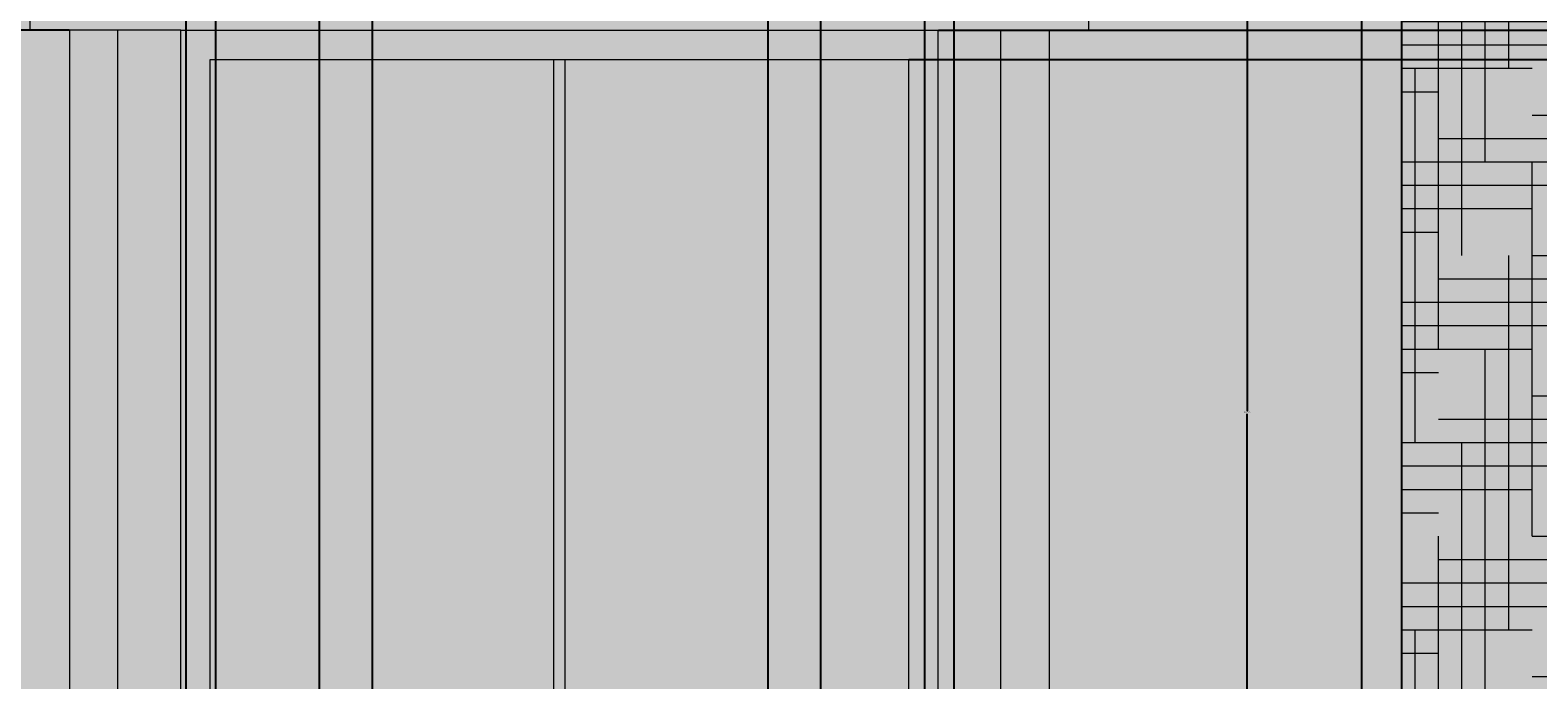
# Model space of a CAD drawing. Units: inches. Extents: x 3024 to 4744, y 1110 to 2100.
# Tile 23 of 29: x 3149 to 3354, y 1809 to 1897. Entities that reach past the tile are written whole.
import ezdxf

# ---------------------------------------------------------------- set-up
doc = ezdxf.new("R2010")
doc.units = ezdxf.units.IN
for name, color, linetype, lineweight in [('A-ANNO-DIMS', 2, 'Continuous', 18), ('A-ELEV', 7, 'Continuous', 25), ('A-ELEV-PATT', 252, 'Continuous', 13), ('A-GLAZ', 4, 'Continuous', 18)]:
    doc.layers.add(name, color=color, linetype=linetype, lineweight=lineweight)
doc.styles.get("Standard").update_dxf_attribs({"font": 'arial.ttf'})
doc.dimstyles.get("Standard").update_dxf_attribs({"dimtxt": 0.18, "dimasz": 0.18, "dimexe": 0.18, "dimexo": 0.0625, "dimgap": 0.09, "dimtad": 0, "dimtih": 1, "dimtoh": 1, "dimdec": 1, "dimzin": 0, "dimdsep": 46, "dimlunit": 3, "dimtxsty": 'Standard', "dimcen": 0.09, "dimadec": 0, "dimazin": 0, "dimtfac": 1, "dimtdec": 1, "dimtofl": 0, "dimtmove": 0, "dimatfit": 3, "dimfxl": 1, "dimtolj": 1, "dimtzin": 0, "dimarcsym": 0})

# ---------------------------------------------------------------- blocks, each defined once
blk = doc.blocks.new('WIN-BALCONY-A')
for p, q in [((3169.4, 1897.49), (3148.97, 1897.49)), ((3169.4, 1897.49), (3148.97, 1897.49)), ((3169.4, 1897.49), (3292.61, 1897.49)), ((3169.4, 1897.49), (3292.61, 1897.49)), ((3169.4, 1795.04), (3148.97, 1795.04)), ((3169.4, 1795.04), (3148.97, 1795.04)), ((3169.4, 1795.04), (3292.61, 1795.04)), ((3169.4, 1795.04), (3292.61, 1795.04))]:
    blk.add_line(p, q)
for points in [[(3148.97, 1897.49), (3148.97, 1905.61), (3292.61, 1905.61), (3292.61, 1897.49)], [(3148.97, 1897.49), (3148.97, 1905.61), (3292.61, 1905.61), (3292.61, 1897.49)], [(3292.61, 1795.04), (3292.61, 1785.61), (3148.97, 1785.61), (3148.97, 1795.04)], [(3292.61, 1795.04), (3292.61, 1785.61), (3148.97, 1785.61), (3148.97, 1795.04)]]:
    blk.add_lwpolyline(points)
for points in [[(3154.33, 1806.87), (3160.86, 1806.87), (3160.86, 1897.49), (3154.33, 1897.49)], [(3154.33, 1806.87), (3160.86, 1806.87), (3160.86, 1897.49), (3154.33, 1897.49)], [(3272.18, 1795.04), (3169.4, 1795.04), (3169.4, 1897.49), (3272.18, 1897.49)], [(3272.18, 1795.04), (3169.4, 1795.04), (3169.4, 1897.49), (3272.18, 1897.49)], [(3287.25, 1806.87), (3280.72, 1806.87), (3280.72, 1897.49), (3287.25, 1897.49)], [(3287.25, 1806.87), (3280.72, 1806.87), (3280.72, 1897.49), (3287.25, 1897.49)], [(3268.18, 1799.04), (3173.4, 1799.04), (3173.4, 1893.49), (3268.18, 1893.49)], [(3268.18, 1799.04), (3173.4, 1799.04), (3173.4, 1893.49), (3268.18, 1893.49)], [(3220.05, 1893.49), (3221.52, 1893.49), (3221.52, 1799.04), (3220.05, 1799.04)], [(3220.05, 1893.49), (3221.52, 1893.49), (3221.52, 1799.04), (3220.05, 1799.04)], [(3163.53, 1795.04), (3151.66, 1795.04), (3151.66, 1806.87), (3163.53, 1806.87)], [(3163.53, 1795.04), (3151.66, 1795.04), (3151.66, 1806.87), (3163.53, 1806.87)], [(3276.51, 1795.04), (3288.38, 1795.04), (3288.38, 1806.87), (3276.51, 1806.87)], [(3276.51, 1795.04), (3288.38, 1795.04), (3288.38, 1806.87), (3276.51, 1806.87)]]:
    blk.add_lwpolyline(points, close=True)
blk = doc.blocks.new('*D7')
at = {"layer": 'A-ANNO-DIMS', "color": 0, "lineweight": -2, "transparency": 16777216}
for p, q in [((3292.67, 1905.61), (3314.33, 1905.61)), ((3314.15, 1905.43), (3314.15, 1845.79)), ((3314.15, 1785.79), (3314.15, 1845.43)), ((3292.67, 1785.61), (3314.33, 1785.61))]:
    blk.add_line(p, q, dxfattribs=at)
at = {"layer": 'A-ANNO-DIMS', "color": 0, "transparency": 16777216}
for points in [[(3314.12, 1905.43), (3314.18, 1905.43), (3314.15, 1905.61)], [(3314.12, 1785.79), (3314.18, 1785.79), (3314.15, 1785.61)]]:
    blk.add_solid(points, dxfattribs=at)
at = {"layer": 'Defpoints', "color": 0, "transparency": 16777216}
for p in [(3292.61, 1905.61), (3314.15, 1905.61), (3292.61, 1785.61)]:
    blk.add_point(p, dxfattribs=at)
at = {"layer": 'A-ANNO-DIMS', "color": 0, "transparency": 16777216, "insert": (3314.15, 1845.61), "char_height": 0.18, "attachment_point": 5}
blk.add_mtext('\\A1;120 TYP.', dxfattribs=at)
blk = doc.blocks.new('*D64')
at = {"layer": 'A-ANNO-DIMS', "color": 0, "lineweight": -2, "transparency": 16777216}
for p, q in [((3069.79, 1241.5), (3069.79, 2100.44)), ((3069.97, 2100.26), (3405.08, 2100.26)), ((3740.97, 2100.26), (3405.87, 2100.26)), ((3741.15, 1241.5), (3741.15, 2100.44))]:
    blk.add_line(p, q, dxfattribs=at)
at = {"layer": 'A-ANNO-DIMS', "color": 0, "transparency": 16777216}
for points in [[(3069.97, 2100.29), (3069.97, 2100.23), (3069.79, 2100.26)], [(3740.97, 2100.29), (3740.97, 2100.23), (3741.15, 2100.26)]]:
    blk.add_solid(points, dxfattribs=at)
at = {"layer": 'Defpoints', "color": 0, "transparency": 16777216}
for p in [(3741.15, 2100.26), (3069.79, 1241.43), (3741.15, 1241.43)]:
    blk.add_point(p, dxfattribs=at)
at = {"layer": 'A-ANNO-DIMS', "color": 0, "transparency": 16777216, "insert": (3405.47, 2100.26), "char_height": 0.18, "attachment_point": 5}
blk.add_mtext('\\A1;671.4', dxfattribs=at)
blk = doc.blocks.new('*D98')
at = {"layer": 'A-ANNO-DIMS', "color": 0, "lineweight": -2, "transparency": 16777216}
for p, q in [((3154.27, 1897.49), (3024.11, 1897.49)), ((3024.29, 1897.31), (3024.29, 1852.36)), ((3024.29, 1807.05), (3024.29, 1852)), ((3154.27, 1806.87), (3024.11, 1806.87))]:
    blk.add_line(p, q, dxfattribs=at)
at = {"layer": 'A-ANNO-DIMS', "color": 0, "transparency": 16777216}
for points in [[(3024.26, 1897.31), (3024.32, 1897.31), (3024.29, 1897.49)], [(3024.26, 1807.05), (3024.32, 1807.05), (3024.29, 1806.87)]]:
    blk.add_solid(points, dxfattribs=at)
at = {"layer": 'Defpoints', "color": 0, "transparency": 16777216}
for p in [(3024.29, 1897.49), (3154.33, 1897.49), (3154.33, 1806.87)]:
    blk.add_point(p, dxfattribs=at)
at = {"layer": 'A-ANNO-DIMS', "color": 0, "transparency": 16777216, "insert": (3024.29, 1852.18), "char_height": 0.18, "attachment_point": 5}
blk.add_mtext('\\A1;90.62', dxfattribs=at)
blk = doc.blocks.new('*D101')
at = {"layer": 'A-ANNO-DIMS', "color": 0, "lineweight": -2, "transparency": 16777216}
for p, q in [((3268.24, 1893.49), (3786.83, 1893.49)), ((3786.65, 1893.31), (3786.65, 1846.45)), ((3786.65, 1799.22), (3786.65, 1846.08)), ((3268.24, 1799.04), (3786.83, 1799.04))]:
    blk.add_line(p, q, dxfattribs=at)
at = {"layer": 'A-ANNO-DIMS', "color": 0, "transparency": 16777216}
for points in [[(3786.62, 1893.31), (3786.68, 1893.31), (3786.65, 1893.49)], [(3786.62, 1799.22), (3786.68, 1799.22), (3786.65, 1799.04)]]:
    blk.add_solid(points, dxfattribs=at)
at = {"layer": 'Defpoints', "color": 0, "transparency": 16777216}
for p in [(3268.18, 1893.49), (3786.65, 1893.49), (3268.18, 1799.04)]:
    blk.add_point(p, dxfattribs=at)
at = {"layer": 'A-ANNO-DIMS', "color": 0, "transparency": 16777216, "insert": (3786.65, 1846.27), "char_height": 0.18, "attachment_point": 5}
blk.add_mtext('\\A1;94.44', dxfattribs=at)
blk = doc.blocks.new('*D102')
at = {"layer": 'A-ANNO-DIMS', "color": 0, "lineweight": -2, "transparency": 16777216}
for p, q in [((3272.24, 1897.49), (3786.83, 1897.49)), ((3786.65, 1897.31), (3786.65, 1895.67)), ((3786.65, 1893.67), (3786.65, 1895.31)), ((3268.24, 1893.49), (3786.83, 1893.49))]:
    blk.add_line(p, q, dxfattribs=at)
at = {"layer": 'A-ANNO-DIMS', "color": 0, "transparency": 16777216}
for points in [[(3786.62, 1897.31), (3786.68, 1897.31), (3786.65, 1897.49)], [(3786.62, 1893.67), (3786.68, 1893.67), (3786.65, 1893.49)]]:
    blk.add_solid(points, dxfattribs=at)
at = {"layer": 'Defpoints', "color": 0, "transparency": 16777216}
for p in [(3272.18, 1897.49), (3786.65, 1897.49), (3268.18, 1893.49)]:
    blk.add_point(p, dxfattribs=at)
at = {"layer": 'A-ANNO-DIMS', "color": 0, "transparency": 16777216, "insert": (3786.65, 1895.49), "char_height": 0.18, "attachment_point": 5}
blk.add_mtext('\\A1;4.00', dxfattribs=at)
blk = doc.blocks.new('*D106')
at = {"layer": 'A-ANNO-DIMS', "color": 0, "lineweight": -2, "transparency": 16777216}
for p, q in [((3170.16, 1275.67), (3170.16, 2100.44)), ((3170.34, 2100.26), (3171.83, 2100.26)), ((3173.98, 2100.26), (3172.49, 2100.26)), ((3174.16, 1271.67), (3174.16, 2100.44))]:
    blk.add_line(p, q, dxfattribs=at)
at = {"layer": 'A-ANNO-DIMS', "color": 0, "transparency": 16777216}
for points in [[(3170.34, 2100.29), (3170.34, 2100.23), (3170.16, 2100.26)], [(3173.98, 2100.29), (3173.98, 2100.23), (3174.16, 2100.26)]]:
    blk.add_solid(points, dxfattribs=at)
at = {"layer": 'Defpoints', "color": 0, "transparency": 16777216}
for p in [(3174.16, 2100.26), (3170.16, 1275.61), (3174.16, 1271.61)]:
    blk.add_point(p, dxfattribs=at)
at = {"layer": 'A-ANNO-DIMS', "color": 0, "transparency": 16777216, "insert": (3172.16, 2100.26), "char_height": 0.18, "attachment_point": 5}
blk.add_mtext('\\A1;4.00', dxfattribs=at)
blk = doc.blocks.new('*D107')
at = {"layer": 'A-ANNO-DIMS', "color": 0, "lineweight": -2, "transparency": 16777216}
for p, q in [((3174.16, 1271.67), (3174.16, 2100.44)), ((3174.34, 2100.26), (3221.88, 2100.26)), ((3270.21, 2100.26), (3222.67, 2100.26)), ((3270.39, 1271.67), (3270.39, 2100.44))]:
    blk.add_line(p, q, dxfattribs=at)
at = {"layer": 'A-ANNO-DIMS', "color": 0, "transparency": 16777216}
for points in [[(3174.34, 2100.29), (3174.34, 2100.23), (3174.16, 2100.26)], [(3270.21, 2100.29), (3270.21, 2100.23), (3270.39, 2100.26)]]:
    blk.add_solid(points, dxfattribs=at)
at = {"layer": 'Defpoints', "color": 0, "transparency": 16777216}
for p in [(3270.39, 2100.26), (3174.16, 1271.61), (3270.39, 1271.61)]:
    blk.add_point(p, dxfattribs=at)
at = {"layer": 'A-ANNO-DIMS', "color": 0, "transparency": 16777216, "insert": (3222.27, 2100.26), "char_height": 0.18, "attachment_point": 5}
blk.add_mtext('\\A1;96.23', dxfattribs=at)
blk = doc.blocks.new('*D108')
at = {"layer": 'A-ANNO-DIMS', "color": 0, "lineweight": -2, "transparency": 16777216}
for p, q in [((3270.39, 1271.67), (3270.39, 2100.44)), ((3270.57, 2100.26), (3272.06, 2100.26)), ((3274.21, 2100.26), (3272.71, 2100.26)), ((3274.39, 1275.67), (3274.39, 2100.44))]:
    blk.add_line(p, q, dxfattribs=at)
at = {"layer": 'A-ANNO-DIMS', "color": 0, "transparency": 16777216}
for points in [[(3270.57, 2100.29), (3270.57, 2100.23), (3270.39, 2100.26)], [(3274.21, 2100.29), (3274.21, 2100.23), (3274.39, 2100.26)]]:
    blk.add_solid(points, dxfattribs=at)
at = {"layer": 'Defpoints', "color": 0, "transparency": 16777216}
for p in [(3274.39, 2100.26), (3274.39, 1275.61), (3270.39, 1271.61)]:
    blk.add_point(p, dxfattribs=at)
at = {"layer": 'A-ANNO-DIMS', "color": 0, "transparency": 16777216, "insert": (3272.39, 2100.26), "char_height": 0.18, "attachment_point": 5}
blk.add_mtext('\\A1;4.00', dxfattribs=at)
blk = doc.blocks.new('*D124')
at = {"layer": 'A-ANNO-DIMS', "color": 0, "lineweight": -2, "transparency": 16777216}
for p, q in [((3174.16, 1271.67), (3174.16, 2100.44)), ((3174.34, 2100.26), (3180.75, 2100.26)), ((3188.08, 2100.26), (3181.67, 2100.26)), ((3188.26, 1256.29), (3188.26, 2100.44))]:
    blk.add_line(p, q, dxfattribs=at)
at = {"layer": 'A-ANNO-DIMS', "color": 0, "transparency": 16777216}
for points in [[(3174.34, 2100.29), (3174.34, 2100.23), (3174.16, 2100.26)], [(3188.08, 2100.29), (3188.08, 2100.23), (3188.26, 2100.26)]]:
    blk.add_solid(points, dxfattribs=at)
at = {"layer": 'Defpoints', "color": 0, "transparency": 16777216}
for p in [(3188.26, 2100.26), (3174.16, 1271.61), (3188.26, 1256.23)]:
    blk.add_point(p, dxfattribs=at)
at = {"layer": 'A-ANNO-DIMS', "color": 0, "transparency": 16777216, "insert": (3181.21, 2100.26), "char_height": 0.18, "attachment_point": 5}
blk.add_mtext('\\A1;14.098', dxfattribs=at)
blk = doc.blocks.new('*D125')
at = {"layer": 'A-ANNO-DIMS', "color": 0, "lineweight": -2, "transparency": 16777216}
for p, q in [((3188.26, 1256.29), (3188.26, 2100.44)), ((3188.44, 2100.26), (3191.44, 2100.26)), ((3195.23, 2100.26), (3192.22, 2100.26)), ((3195.41, 1256.29), (3195.41, 2100.44))]:
    blk.add_line(p, q, dxfattribs=at)
at = {"layer": 'A-ANNO-DIMS', "color": 0, "transparency": 16777216}
for points in [[(3188.44, 2100.29), (3188.44, 2100.23), (3188.26, 2100.26)], [(3195.23, 2100.29), (3195.23, 2100.23), (3195.41, 2100.26)]]:
    blk.add_solid(points, dxfattribs=at)
at = {"layer": 'Defpoints', "color": 0, "transparency": 16777216}
for p in [(3195.41, 2100.26), (3188.26, 1256.23), (3195.41, 1256.23)]:
    blk.add_point(p, dxfattribs=at)
at = {"layer": 'A-ANNO-DIMS', "color": 0, "transparency": 16777216, "insert": (3191.83, 2100.26), "char_height": 0.18, "attachment_point": 5}
blk.add_mtext('\\A1;7.147', dxfattribs=at)
blk = doc.blocks.new('*D126')
at = {"layer": 'A-ANNO-DIMS', "color": 0, "lineweight": -2, "transparency": 16777216}
for p, q in [((3249.14, 1256.29), (3249.14, 2100.44)), ((3249.32, 2100.26), (3252.32, 2100.26)), ((3256.11, 2100.26), (3253.11, 2100.26)), ((3256.29, 1256.29), (3256.29, 2100.44))]:
    blk.add_line(p, q, dxfattribs=at)
at = {"layer": 'A-ANNO-DIMS', "color": 0, "transparency": 16777216}
for points in [[(3249.32, 2100.29), (3249.32, 2100.23), (3249.14, 2100.26)], [(3256.11, 2100.29), (3256.11, 2100.23), (3256.29, 2100.26)]]:
    blk.add_solid(points, dxfattribs=at)
at = {"layer": 'Defpoints', "color": 0, "transparency": 16777216}
for p in [(3256.29, 2100.26), (3249.14, 1256.23), (3256.29, 1256.23)]:
    blk.add_point(p, dxfattribs=at)
at = {"layer": 'A-ANNO-DIMS', "color": 0, "transparency": 16777216, "insert": (3252.72, 2100.26), "char_height": 0.18, "attachment_point": 5}
blk.add_mtext('\\A1;7.147', dxfattribs=at)

msp = doc.modelspace()

# ---------------------------------------------------------------- hatches: boundary and pattern name
at = {"layer": 'A-ELEV-PATT'}
h = msp.add_hatch(color=256, dxfattribs=at)
h.dxf.hatch_style = 1
h.paths.add_polyline_path([(3491.8271, 2054.7584), (3320.5658, 2054.7584), (3320.5658, 2043.5286), (3491.8271, 2043.5286)])
h.paths.add_polyline_path([(3292.6051, 1905.6112), (3148.9694, 1905.6112), (3148.9694, 1897.4879), (3169.3964, 1897.4879), (3292.6051, 1897.4879)])
h.paths.add_polyline_path([(3292.6051, 1795.0431), (3169.3964, 1795.0431), (3148.9694, 1795.0431), (3148.9694, 1785.6112), (3292.6051, 1785.6112)])
h.paths.add_polyline_path([(3292.6051, 1779.6112), (3148.9694, 1779.6112), (3148.9694, 1771.4879), (3169.3964, 1771.4879), (3292.6051, 1771.4879)])
h.paths.add_polyline_path([(3292.6051, 1669.0431), (3169.3964, 1669.0431), (3148.9694, 1669.0431), (3148.9694, 1659.6112), (3292.6051, 1659.6112)])
h.paths.add_polyline_path([(3292.6051, 1653.6112), (3148.9694, 1653.6112), (3148.9694, 1645.4879), (3169.3964, 1645.4879), (3292.6051, 1645.4879)])
h.paths.add_polyline_path([(3292.6051, 1543.0431), (3169.3964, 1543.0431), (3148.9694, 1543.0431), (3148.9694, 1533.6112), (3292.6051, 1533.6112)])
h.paths.add_polyline_path([(3292.6051, 1527.6112), (3148.9694, 1527.6112), (3148.9694, 1519.4879), (3169.3964, 1519.4879), (3292.6051, 1519.4879)])
h.paths.add_polyline_path([(3292.6051, 1401.6112), (3148.9694, 1401.6112), (3148.9694, 1393.4879), (3169.3964, 1393.4879), (3292.6051, 1393.4879)])
h.paths.add_polyline_path([(3292.6051, 1417.0431), (3169.3964, 1417.0431), (3148.9694, 1417.0431), (3148.9694, 1407.6112), (3292.6051, 1407.6112)])
h.paths.add_polyline_path([(3292.6051, 1291.0431), (3169.3964, 1291.0431), (3148.9694, 1291.0431), (3148.9694, 1281.6112), (3292.6051, 1281.6112)])
h.paths.add_polyline_path([(3654.037, 1165.0431), (3530.8283, 1165.0431), (3510.4013, 1165.0431), (3510.4013, 1155.6112), (3654.037, 1155.6112)])
h.paths.add_polyline_path([(3654.037, 1275.6112), (3510.4013, 1275.6112), (3510.4013, 1267.4879), (3530.8283, 1267.4879), (3654.037, 1267.4879)])
h.paths.add_polyline_path([(3654.037, 1291.0431), (3530.8283, 1291.0431), (3510.4013, 1291.0431), (3510.4013, 1281.6112), (3654.037, 1281.6112)])
h.paths.add_polyline_path([(3654.037, 1417.0431), (3530.8283, 1417.0431), (3510.4013, 1417.0431), (3510.4013, 1407.6112), (3654.037, 1407.6112)])
h.paths.add_polyline_path([(3654.037, 1401.6112), (3510.4013, 1401.6112), (3510.4013, 1393.4879), (3530.8283, 1393.4879), (3654.037, 1393.4879)])
h.paths.add_polyline_path([(3654.037, 1543.0431), (3530.8283, 1543.0431), (3510.4013, 1543.0431), (3510.4013, 1533.6112), (3654.037, 1533.6112)])
h.paths.add_polyline_path([(3654.037, 1527.6112), (3510.4013, 1527.6112), (3510.4013, 1519.4879), (3530.8283, 1519.4879), (3654.037, 1519.4879)])
h.paths.add_polyline_path([(3654.037, 1653.6112), (3510.4013, 1653.6112), (3510.4013, 1645.4879), (3530.8283, 1645.4879), (3654.037, 1645.4879)])
h.paths.add_polyline_path([(3654.037, 1669.0431), (3530.8283, 1669.0431), (3510.4013, 1669.0431), (3510.4013, 1659.6112), (3654.037, 1659.6112)])
h.paths.add_polyline_path([(3654.037, 1779.6112), (3510.4013, 1779.6112), (3510.4013, 1771.4879), (3530.8283, 1771.4879), (3654.037, 1771.4879)])
h.paths.add_polyline_path([(3654.037, 1795.0431), (3530.8283, 1795.0431), (3510.4013, 1795.0431), (3510.4013, 1785.6112), (3654.037, 1785.6112)])
h.paths.add_polyline_path([(3654.037, 1905.6112), (3510.4013, 1905.6112), (3510.4013, 1897.4879), (3530.8283, 1897.4879), (3654.037, 1897.4879)])
h = msp.add_hatch(color=256, dxfattribs=at)
h.dxf.hatch_style = 1
h.paths.add_polyline_path([(3335.1044, 2043.5286), (3329.7033, 2043.5286), (3329.7033, 1155.6112), (3335.1044, 1155.6112)])
h.paths.add_polyline_path([(3481.2411, 2043.5286), (3335.1044, 2043.5286), (3335.1044, 1155.6112), (3481.2411, 1155.6112)])
h.paths.add_polyline_path([(3449.7202, 1329.5246), (3361.2242, 1329.5246), (3361.2242, 1436.6064), (3449.7202, 1436.6064)], flags=16)
h.paths.add_polyline_path([(3445.7202, 1333.5246), (3365.2242, 1333.5246), (3365.2242, 1432.6064), (3445.7202, 1432.6064)], flags=0)
h.paths.add_polyline_path([(3449.7202, 1455.5246), (3361.2242, 1455.5246), (3361.2242, 1562.6064), (3449.7202, 1562.6064)], flags=16)
h.paths.add_polyline_path([(3445.7202, 1459.5246), (3365.2242, 1459.5246), (3365.2242, 1558.6064), (3445.7202, 1558.6064)], flags=0)
h.paths.add_polyline_path([(3449.7202, 1581.5246), (3361.2242, 1581.5246), (3361.2242, 1688.6064), (3449.7202, 1688.6064)], flags=16)
h.paths.add_polyline_path([(3445.7202, 1585.5246), (3365.2242, 1585.5246), (3365.2242, 1684.6064), (3445.7202, 1684.6064)], flags=0)
h.paths.add_polyline_path([(3449.7202, 1707.5246), (3361.2242, 1707.5246), (3361.2242, 1814.6064), (3449.7202, 1814.6064)], flags=16)
h.paths.add_polyline_path([(3445.7202, 1711.5246), (3365.2242, 1711.5246), (3365.2242, 1810.6064), (3445.7202, 1810.6064)], flags=0)
h.paths.add_polyline_path([(3449.7202, 1833.5246), (3361.2242, 1833.5246), (3361.2242, 1940.6064), (3449.7202, 1940.6064)], flags=16)
h.paths.add_polyline_path([(3445.7202, 1837.5246), (3365.2242, 1837.5246), (3365.2242, 1936.6064), (3445.7202, 1936.6064)], flags=0)
h = msp.add_hatch(color=256, dxfattribs=at)
h.dxf.hatch_style = 1
h.paths.add_polyline_path([(3475.84, 2043.5286), (3335.1044, 2043.5286), (3335.1044, 1155.6112), (3475.84, 1155.6112)])
h.paths.add_polyline_path([(3449.7202, 1940.6064), (3449.7202, 1833.5246), (3361.2242, 1833.5246), (3361.2242, 1940.6064)], flags=16)
h.paths.add_polyline_path([(3445.7202, 1936.6064), (3445.7202, 1837.5246), (3365.2242, 1837.5246), (3365.2242, 1936.6064)], flags=0)
h.paths.add_polyline_path([(3449.7202, 1814.6064), (3449.7202, 1707.5246), (3361.2242, 1707.5246), (3361.2242, 1814.6064)], flags=16)
h.paths.add_polyline_path([(3445.7202, 1810.6064), (3445.7202, 1711.5246), (3365.2242, 1711.5246), (3365.2242, 1810.6064)], flags=0)
h.paths.add_polyline_path([(3449.7202, 1688.6064), (3449.7202, 1581.5246), (3361.2242, 1581.5246), (3361.2242, 1688.6064)], flags=16)
h.paths.add_polyline_path([(3445.7202, 1684.6064), (3445.7202, 1585.5246), (3365.2242, 1585.5246), (3365.2242, 1684.6064)], flags=0)
h.paths.add_polyline_path([(3449.7202, 1562.6064), (3449.7202, 1455.5246), (3361.2242, 1455.5246), (3361.2242, 1562.6064)], flags=16)
h.paths.add_polyline_path([(3445.7202, 1558.6064), (3445.7202, 1459.5246), (3365.2242, 1459.5246), (3365.2242, 1558.6064)], flags=0)
h.paths.add_polyline_path([(3449.7202, 1436.6064), (3449.7202, 1329.5246), (3361.2242, 1329.5246), (3361.2242, 1436.6064)], flags=16)
h.paths.add_polyline_path([(3445.7202, 1432.6064), (3445.7202, 1333.5246), (3365.2242, 1333.5246), (3365.2242, 1432.6064)], flags=0)
h = msp.add_hatch(dxfattribs=at)
h.set_pattern_fill('HOUND', color=256, scale=2)
h.paths.add_polyline_path([(3475.84, 2043.5286), (3335.1044, 2043.5286), (3335.1044, 1155.6112), (3475.84, 1155.6112)])
h.paths.add_polyline_path([(3449.7202, 1940.6064), (3449.7202, 1833.5246), (3361.2242, 1833.5246), (3361.2242, 1940.6064)], flags=16)
h.paths.add_polyline_path([(3445.7202, 1936.6064), (3445.7202, 1837.5246), (3365.2242, 1837.5246), (3365.2242, 1936.6064)], flags=0)
h.paths.add_polyline_path([(3449.7202, 1814.6064), (3449.7202, 1707.5246), (3361.2242, 1707.5246), (3361.2242, 1814.6064)], flags=16)
h.paths.add_polyline_path([(3445.7202, 1810.6064), (3445.7202, 1711.5246), (3365.2242, 1711.5246), (3365.2242, 1810.6064)], flags=0)
h.paths.add_polyline_path([(3449.7202, 1688.6064), (3449.7202, 1581.5246), (3361.2242, 1581.5246), (3361.2242, 1688.6064)], flags=16)
h.paths.add_polyline_path([(3445.7202, 1684.6064), (3445.7202, 1585.5246), (3365.2242, 1585.5246), (3365.2242, 1684.6064)], flags=0)
h.paths.add_polyline_path([(3449.7202, 1562.6064), (3449.7202, 1455.5246), (3361.2242, 1455.5246), (3361.2242, 1562.6064)], flags=16)
h.paths.add_polyline_path([(3445.7202, 1558.6064), (3445.7202, 1459.5246), (3365.2242, 1459.5246), (3365.2242, 1558.6064)], flags=0)
h.paths.add_polyline_path([(3449.7202, 1436.6064), (3449.7202, 1329.5246), (3361.2242, 1329.5246), (3361.2242, 1436.6064)], flags=16)
h.paths.add_polyline_path([(3445.7202, 1432.6064), (3445.7202, 1333.5246), (3365.2242, 1333.5246), (3365.2242, 1432.6064)], flags=0)
h = msp.add_hatch(color=256, dxfattribs=at)
h.dxf.hatch_style = 1
h.paths.add_polyline_path([(3221.5241, 2019.4879), (3220.0505, 2019.4879), (3220.0505, 1925.0431), (3221.5241, 1925.0431)], flags=0)
h.paths.add_polyline_path([(3221.5241, 2019.4879), (3221.5241, 1925.0431), (3220.0505, 1925.0431), (3220.0505, 2019.4879)], flags=0)
h.paths.add_polyline_path([(3221.5241, 1893.4879), (3220.0505, 1893.4879), (3220.0505, 1799.0431), (3221.5241, 1799.0431)])
h = msp.add_hatch(color=256, dxfattribs=at)
h.dxf.hatch_style = 1
h.paths.add_polyline_path([(3154.3287, 1897.4879), (3148.9694, 1897.4879), (3148.9694, 1905.6112), (3105.4722, 1905.6112), (3105.4722, 1785.6112), (3148.9694, 1785.6112), (3148.9694, 1795.0431), (3151.6604, 1795.0431), (3151.6604, 1806.8674), (3154.3287, 1806.8674)])
h.paths.add_polyline_path([(3329.7033, 1905.6112), (3292.6051, 1905.6112), (3292.6051, 1897.4879), (3287.2458, 1897.4879), (3287.2458, 1806.8674), (3288.3759, 1806.8674), (3288.3759, 1795.0431), (3292.6051, 1795.0431), (3292.6051, 1785.6112), (3329.7033, 1785.6112)])
h.paths.add_polyline_path([(3154.3287, 1771.4879), (3148.9694, 1771.4879), (3148.9694, 1779.6112), (3105.4722, 1779.6112), (3105.4722, 1659.6112), (3148.9694, 1659.6112), (3148.9694, 1669.0431), (3151.6604, 1669.0431), (3151.6604, 1680.8674), (3154.3287, 1680.8674)])
h.paths.add_polyline_path([(3329.7033, 1779.6112), (3292.6051, 1779.6112), (3292.6051, 1771.4879), (3287.2458, 1771.4879), (3287.2458, 1680.8674), (3288.3759, 1680.8674), (3288.3759, 1669.0431), (3292.6051, 1669.0431), (3292.6051, 1659.6112), (3329.7033, 1659.6112)])
h.paths.add_polyline_path([(3154.3287, 1645.4879), (3148.9694, 1645.4879), (3148.9694, 1653.6112), (3105.4722, 1653.6112), (3105.4722, 1533.6112), (3148.9694, 1533.6112), (3148.9694, 1543.0431), (3151.6604, 1543.0431), (3151.6604, 1554.8674), (3154.3287, 1554.8674)])
h.paths.add_polyline_path([(3329.7033, 1653.6112), (3292.6051, 1653.6112), (3292.6051, 1645.4879), (3287.2458, 1645.4879), (3287.2458, 1554.8674), (3288.3759, 1554.8674), (3288.3759, 1543.0431), (3292.6051, 1543.0431), (3292.6051, 1533.6112), (3329.7033, 1533.6112)])
h.paths.add_polyline_path([(3329.7033, 1527.6112), (3292.6051, 1527.6112), (3292.6051, 1519.4879), (3287.2458, 1519.4879), (3287.2458, 1428.8674), (3288.3759, 1428.8674), (3288.3759, 1417.0431), (3292.6051, 1417.0431), (3292.6051, 1407.6112), (3329.7033, 1407.6112)])
h.paths.add_polyline_path([(3329.7033, 1401.6112), (3292.6051, 1401.6112), (3292.6051, 1393.4879), (3287.2458, 1393.4879), (3287.2458, 1302.8674), (3288.3759, 1302.8674), (3288.3759, 1291.0431), (3292.6051, 1291.0431), (3292.6051, 1281.6112), (3329.7033, 1281.6112)])
h.paths.add_polyline_path([(3154.3287, 1393.4879), (3148.9694, 1393.4879), (3148.9694, 1401.6112), (3105.4722, 1401.6112), (3105.4722, 1281.6112), (3148.9694, 1281.6112), (3148.9694, 1291.0431), (3151.6604, 1291.0431), (3151.6604, 1302.8674), (3154.3287, 1302.8674)])
h.paths.add_polyline_path([(3154.3287, 1519.4879), (3148.9694, 1519.4879), (3148.9694, 1527.6112), (3105.4722, 1527.6112), (3105.4722, 1407.6112), (3148.9694, 1407.6112), (3148.9694, 1417.0431), (3151.6604, 1417.0431), (3151.6604, 1428.8674), (3154.3287, 1428.8674)])
h.paths.add_polyline_path([(3515.7606, 1897.4879), (3510.4013, 1897.4879), (3510.4013, 1905.6112), (3481.2411, 1905.6112), (3481.2411, 1785.6112), (3510.4013, 1785.6112), (3510.4013, 1795.0431), (3513.0923, 1795.0431), (3513.0923, 1806.8674), (3515.7606, 1806.8674)])
h.paths.add_polyline_path([(3688.5588, 1905.6112), (3654.037, 1905.6112), (3654.037, 1897.4879), (3648.6777, 1897.4879), (3648.6777, 1806.8674), (3649.8078, 1806.8674), (3649.8078, 1795.0431), (3654.037, 1795.0431), (3654.037, 1785.6112), (3688.5588, 1785.6112)])
h.paths.add_polyline_path([(3515.7606, 1771.4879), (3510.4013, 1771.4879), (3510.4013, 1779.6112), (3481.2411, 1779.6112), (3481.2411, 1659.6112), (3510.4013, 1659.6112), (3510.4013, 1669.0431), (3513.0923, 1669.0431), (3513.0923, 1680.8674), (3515.7606, 1680.8674)])
h.paths.add_polyline_path([(3688.5588, 1779.6112), (3654.037, 1779.6112), (3654.037, 1771.4879), (3648.6777, 1771.4879), (3648.6777, 1680.8674), (3649.8078, 1680.8674), (3649.8078, 1669.0431), (3654.037, 1669.0431), (3654.037, 1659.6112), (3688.5588, 1659.6112)])
h.paths.add_polyline_path([(3515.7606, 1645.4879), (3510.4013, 1645.4879), (3510.4013, 1653.6112), (3481.2411, 1653.6112), (3481.2411, 1533.6112), (3510.4013, 1533.6112), (3510.4013, 1543.0431), (3513.0923, 1543.0431), (3513.0923, 1554.8674), (3515.7606, 1554.8674)])
h.paths.add_polyline_path([(3688.5588, 1653.6112), (3654.037, 1653.6112), (3654.037, 1645.4879), (3648.6777, 1645.4879), (3648.6777, 1554.8674), (3649.8078, 1554.8674), (3649.8078, 1543.0431), (3654.037, 1543.0431), (3654.037, 1533.6112), (3688.5588, 1533.6112)])
h.paths.add_polyline_path([(3515.7606, 1519.4879), (3510.4013, 1519.4879), (3510.4013, 1527.6112), (3481.2411, 1527.6112), (3481.2411, 1407.6112), (3510.4013, 1407.6112), (3510.4013, 1417.0431), (3513.0923, 1417.0431), (3513.0923, 1428.8674), (3515.7606, 1428.8674)])
h.paths.add_polyline_path([(3688.5588, 1527.6112), (3654.037, 1527.6112), (3654.037, 1519.4879), (3648.6777, 1519.4879), (3648.6777, 1428.8674), (3649.8078, 1428.8674), (3649.8078, 1417.0431), (3654.037, 1417.0431), (3654.037, 1407.6112), (3688.5588, 1407.6112)])
h.paths.add_polyline_path([(3515.7606, 1393.4879), (3510.4013, 1393.4879), (3510.4013, 1401.6112), (3481.2411, 1401.6112), (3481.2411, 1281.6112), (3510.4013, 1281.6112), (3510.4013, 1291.0431), (3513.0923, 1291.0431), (3513.0923, 1302.8674), (3515.7606, 1302.8674)])
h.paths.add_polyline_path([(3688.5588, 1401.6112), (3654.037, 1401.6112), (3654.037, 1393.4879), (3648.6777, 1393.4879), (3648.6777, 1302.8674), (3649.8078, 1302.8674), (3649.8078, 1291.0431), (3654.037, 1291.0431), (3654.037, 1281.6112), (3688.5588, 1281.6112)])
h.paths.add_polyline_path([(3515.7606, 1267.4879), (3510.4013, 1267.4879), (3510.4013, 1275.6112), (3481.2411, 1275.6112), (3481.2411, 1155.6112), (3510.4013, 1155.6112), (3510.4013, 1165.0431), (3513.0923, 1165.0431), (3513.0923, 1176.8674), (3515.7606, 1176.8674)])
h.paths.add_polyline_path([(3688.5588, 1275.6112), (3654.037, 1275.6112), (3654.037, 1267.4879), (3648.6777, 1267.4879), (3648.6777, 1176.8674), (3649.8078, 1176.8674), (3649.8078, 1165.0431), (3654.037, 1165.0431), (3654.037, 1155.6112), (3688.5588, 1155.6112)])
h.paths.add_polyline_path([(3112.3838, 1275.6112), (3105.4722, 1275.6112), (3105.4722, 1171.0239), (3112.3838, 1171.0239)])
h = msp.add_hatch(color=256, dxfattribs=at)
h.dxf.hatch_style = 1
h.paths.add_polyline_path([(3160.8586, 1897.4879), (3154.3287, 1897.4879), (3154.3287, 1806.8674), (3160.8586, 1806.8674)])
h.paths.add_polyline_path([(3287.2458, 1897.4879), (3280.716, 1897.4879), (3280.716, 1806.8674), (3287.2458, 1806.8674)])
h.paths.add_polyline_path([(3160.8586, 1771.4879), (3154.3287, 1771.4879), (3154.3287, 1680.8674), (3160.8586, 1680.8674)])
h.paths.add_polyline_path([(3287.2458, 1771.4879), (3280.716, 1771.4879), (3280.716, 1680.8674), (3287.2458, 1680.8674)])
h.paths.add_polyline_path([(3160.8586, 1645.4879), (3154.3287, 1645.4879), (3154.3287, 1554.8674), (3160.8586, 1554.8674)])
h.paths.add_polyline_path([(3287.2458, 1645.4879), (3280.716, 1645.4879), (3280.716, 1554.8674), (3287.2458, 1554.8674)])
h.paths.add_polyline_path([(3160.8586, 1519.4879), (3154.3287, 1519.4879), (3154.3287, 1428.8674), (3160.8586, 1428.8674)])
h.paths.add_polyline_path([(3287.2458, 1519.4879), (3280.716, 1519.4879), (3280.716, 1428.8674), (3287.2458, 1428.8674)])
h.paths.add_polyline_path([(3160.8586, 1393.4879), (3154.3287, 1393.4879), (3154.3287, 1302.8674), (3160.8586, 1302.8674)])
h.paths.add_polyline_path([(3287.2458, 1393.4879), (3280.716, 1393.4879), (3280.716, 1302.8674), (3287.2458, 1302.8674)])
h.paths.add_polyline_path([(3648.6777, 1267.4879), (3642.1479, 1267.4879), (3642.1479, 1176.8674), (3648.6777, 1176.8674)])
h.paths.add_polyline_path([(3522.2905, 1267.4879), (3515.7606, 1267.4879), (3515.7606, 1176.8674), (3522.2905, 1176.8674)])
h.paths.add_polyline_path([(3522.2905, 1393.4879), (3515.7606, 1393.4879), (3515.7606, 1302.8674), (3522.2905, 1302.8674)])
h.paths.add_polyline_path([(3648.6777, 1393.4879), (3642.1479, 1393.4879), (3642.1479, 1302.8674), (3648.6777, 1302.8674)])
h.paths.add_polyline_path([(3522.2905, 1519.4879), (3515.7606, 1519.4879), (3515.7606, 1428.8674), (3522.2905, 1428.8674)])
h.paths.add_polyline_path([(3648.6777, 1519.4879), (3642.1479, 1519.4879), (3642.1479, 1428.8674), (3648.6777, 1428.8674)])
h.paths.add_polyline_path([(3522.2905, 1645.4879), (3515.7606, 1645.4879), (3515.7606, 1554.8674), (3522.2905, 1554.8674)])
h.paths.add_polyline_path([(3522.2905, 1771.4879), (3515.7606, 1771.4879), (3515.7606, 1680.8674), (3522.2905, 1680.8674)])
h.paths.add_polyline_path([(3648.6777, 1645.4879), (3642.1479, 1645.4879), (3642.1479, 1554.8674), (3648.6777, 1554.8674)])
h.paths.add_polyline_path([(3648.6777, 1771.4879), (3642.1479, 1771.4879), (3642.1479, 1680.8674), (3648.6777, 1680.8674)])
h.paths.add_polyline_path([(3648.6777, 1897.4879), (3642.1479, 1897.4879), (3642.1479, 1806.8674), (3648.6777, 1806.8674)])
h.paths.add_polyline_path([(3522.2905, 1897.4879), (3515.7606, 1897.4879), (3515.7606, 1806.8674), (3522.2905, 1806.8674)])
h = msp.add_hatch(color=256, dxfattribs=at)
h.dxf.hatch_style = 1
h.paths.add_polyline_path([(3169.3964, 1897.4879), (3160.8586, 1897.4879), (3160.8586, 1806.8674), (3163.5269, 1806.8674), (3163.5269, 1795.0431), (3169.3964, 1795.0431)])
h.paths.add_polyline_path([(3280.716, 1897.4879), (3272.1781, 1897.4879), (3272.1781, 1795.0431), (3276.5094, 1795.0431), (3276.5094, 1806.8674), (3280.716, 1806.8674)])
h.paths.add_polyline_path([(3280.716, 1771.4879), (3272.1781, 1771.4879), (3272.1781, 1669.0431), (3276.5094, 1669.0431), (3276.5094, 1680.8674), (3280.716, 1680.8674)])
h.paths.add_polyline_path([(3169.3964, 1771.4879), (3160.8586, 1771.4879), (3160.8586, 1680.8674), (3163.5269, 1680.8674), (3163.5269, 1669.0431), (3169.3964, 1669.0431)])
h.paths.add_polyline_path([(3169.3964, 1645.4879), (3160.8586, 1645.4879), (3160.8586, 1554.8674), (3163.5269, 1554.8674), (3163.5269, 1543.0431), (3169.3964, 1543.0431)])
h.paths.add_polyline_path([(3280.716, 1645.4879), (3272.1781, 1645.4879), (3272.1781, 1543.0431), (3276.5094, 1543.0431), (3276.5094, 1554.8674), (3280.716, 1554.8674)])
h.paths.add_polyline_path([(3169.3964, 1519.4879), (3160.8586, 1519.4879), (3160.8586, 1428.8674), (3163.5269, 1428.8674), (3163.5269, 1417.0431), (3169.3964, 1417.0431)])
h.paths.add_polyline_path([(3280.716, 1519.4879), (3272.1781, 1519.4879), (3272.1781, 1417.0431), (3276.5094, 1417.0431), (3276.5094, 1428.8674), (3280.716, 1428.8674)])
h.paths.add_polyline_path([(3169.3964, 1393.4879), (3160.8586, 1393.4879), (3160.8586, 1302.8674), (3163.5269, 1302.8674), (3163.5269, 1291.0431), (3169.3964, 1291.0431)])
h.paths.add_polyline_path([(3280.716, 1393.4879), (3272.1781, 1393.4879), (3272.1781, 1291.0431), (3276.5094, 1291.0431), (3276.5094, 1302.8674), (3280.716, 1302.8674)])
h.paths.add_polyline_path([(3642.1479, 1267.4879), (3633.61, 1267.4879), (3633.61, 1165.0431), (3637.9413, 1165.0431), (3637.9413, 1176.8674), (3642.1479, 1176.8674)])
h.paths.add_polyline_path([(3530.8283, 1267.4879), (3522.2905, 1267.4879), (3522.2905, 1176.8674), (3524.9588, 1176.8674), (3524.9588, 1165.0431), (3530.8283, 1165.0431)])
h.paths.add_polyline_path([(3642.1479, 1393.4879), (3633.61, 1393.4879), (3633.61, 1291.0431), (3637.9413, 1291.0431), (3637.9413, 1302.8674), (3642.1479, 1302.8674)])
h.paths.add_polyline_path([(3530.8283, 1393.4879), (3522.2905, 1393.4879), (3522.2905, 1302.8674), (3524.9588, 1302.8674), (3524.9588, 1291.0431), (3530.8283, 1291.0431)])
h.paths.add_polyline_path([(3530.8283, 1519.4879), (3522.2905, 1519.4879), (3522.2905, 1428.8674), (3524.9588, 1428.8674), (3524.9588, 1417.0431), (3530.8283, 1417.0431)])
h.paths.add_polyline_path([(3642.1479, 1519.4879), (3633.61, 1519.4879), (3633.61, 1417.0431), (3637.9413, 1417.0431), (3637.9413, 1428.8674), (3642.1479, 1428.8674)])
h.paths.add_polyline_path([(3530.8283, 1645.4879), (3522.2905, 1645.4879), (3522.2905, 1554.8674), (3524.9588, 1554.8674), (3524.9588, 1543.0431), (3530.8283, 1543.0431)])
h.paths.add_polyline_path([(3642.1479, 1645.4879), (3633.61, 1645.4879), (3633.61, 1543.0431), (3637.9413, 1543.0431), (3637.9413, 1554.8674), (3642.1479, 1554.8674)])
h.paths.add_polyline_path([(3642.1479, 1771.4879), (3633.61, 1771.4879), (3633.61, 1669.0431), (3637.9413, 1669.0431), (3637.9413, 1680.8674), (3642.1479, 1680.8674)])
h.paths.add_polyline_path([(3530.8283, 1771.4879), (3522.2905, 1771.4879), (3522.2905, 1680.8674), (3524.9588, 1680.8674), (3524.9588, 1669.0431), (3530.8283, 1669.0431)])
h.paths.add_polyline_path([(3530.8283, 1897.4879), (3522.2905, 1897.4879), (3522.2905, 1806.8674), (3524.9588, 1806.8674), (3524.9588, 1795.0431), (3530.8283, 1795.0431)])
h.paths.add_polyline_path([(3642.1479, 1897.4879), (3633.61, 1897.4879), (3633.61, 1795.0431), (3637.9413, 1795.0431), (3637.9413, 1806.8674), (3642.1479, 1806.8674)])
h = msp.add_hatch(color=256, dxfattribs=at)
h.dxf.hatch_style = 1
h.paths.add_polyline_path([(3221.5241, 1893.4879), (3220.0505, 1893.4879), (3220.0505, 1799.0431), (3221.5241, 1799.0431)], flags=0)
h.paths.add_polyline_path([(3272.1781, 1897.4879), (3169.3964, 1897.4879), (3169.3964, 1795.0431), (3272.1781, 1795.0431)])
h.paths.add_polyline_path([(3268.1781, 1893.4879), (3268.1781, 1799.0431), (3173.3964, 1799.0431), (3173.3964, 1893.4879)], flags=16)
h.paths.add_polyline_path([(3221.5241, 1893.4879), (3221.5241, 1799.0431), (3220.0505, 1799.0431), (3220.0505, 1893.4879)], flags=0)
h = msp.add_hatch(color=256, dxfattribs=at)
h.dxf.hatch_style = 1
h.paths.add_polyline_path([(3220.0505, 1893.4879), (3173.3964, 1893.4879), (3173.3964, 1799.0431), (3220.0505, 1799.0431)])
h.paths.add_polyline_path([(3268.1781, 1893.4879), (3221.5241, 1893.4879), (3221.5241, 1799.0431), (3268.1781, 1799.0431)])
h.paths.add_polyline_path([(3581.4824, 1893.4879), (3534.8283, 1893.4879), (3534.8283, 1799.0431), (3581.4824, 1799.0431)])
h.paths.add_polyline_path([(3629.61, 1893.4879), (3582.956, 1893.4879), (3582.956, 1799.0431), (3629.61, 1799.0431)])
h.paths.add_polyline_path([(3581.4824, 1767.4879), (3534.8283, 1767.4879), (3534.8283, 1673.0431), (3581.4824, 1673.0431)])
h.paths.add_polyline_path([(3629.61, 1767.4879), (3582.956, 1767.4879), (3582.956, 1673.0431), (3629.61, 1673.0431)])
h.paths.add_polyline_path([(3581.4824, 1641.4879), (3534.8283, 1641.4879), (3534.8283, 1547.0431), (3581.4824, 1547.0431)])
h.paths.add_polyline_path([(3629.61, 1641.4879), (3582.956, 1641.4879), (3582.956, 1547.0431), (3629.61, 1547.0431)])
h.paths.add_polyline_path([(3629.61, 1515.4879), (3582.956, 1515.4879), (3582.956, 1421.0431), (3629.61, 1421.0431)])
h.paths.add_polyline_path([(3581.4824, 1515.4879), (3534.8283, 1515.4879), (3534.8283, 1421.0431), (3581.4824, 1421.0431)])
h.paths.add_polyline_path([(3629.61, 1389.4879), (3582.956, 1389.4879), (3582.956, 1295.0431), (3629.61, 1295.0431)])
h.paths.add_polyline_path([(3581.4824, 1389.4879), (3534.8283, 1389.4879), (3534.8283, 1295.0431), (3581.4824, 1295.0431)])
h.paths.add_polyline_path([(3629.61, 1263.4879), (3582.956, 1263.4879), (3582.956, 1169.0431), (3629.61, 1169.0431)])
h.paths.add_polyline_path([(3581.4824, 1263.4879), (3534.8283, 1263.4879), (3534.8283, 1169.0431), (3581.4824, 1169.0431)])
h.paths.add_polyline_path([(3220.0505, 1389.4879), (3173.3964, 1389.4879), (3173.3964, 1295.0431), (3220.0505, 1295.0431)])
h.paths.add_polyline_path([(3268.1781, 1389.4879), (3221.5241, 1389.4879), (3221.5241, 1295.0431), (3268.1781, 1295.0431)])
h.paths.add_polyline_path([(3220.0505, 1515.4879), (3173.3964, 1515.4879), (3173.3964, 1421.0431), (3220.0505, 1421.0431)])
h.paths.add_polyline_path([(3268.1781, 1515.4879), (3221.5241, 1515.4879), (3221.5241, 1421.0431), (3268.1781, 1421.0431)])
h.paths.add_polyline_path([(3220.0505, 1767.4879), (3173.3964, 1767.4879), (3173.3964, 1673.0431), (3220.0505, 1673.0431)])
h.paths.add_polyline_path([(3268.1781, 1767.4879), (3221.5241, 1767.4879), (3221.5241, 1673.0431), (3268.1781, 1673.0431)])
h.paths.add_polyline_path([(3220.0505, 1641.4879), (3173.3964, 1641.4879), (3173.3964, 1547.0431), (3220.0505, 1547.0431)])
h.paths.add_polyline_path([(3268.1781, 1641.4879), (3221.5241, 1641.4879), (3221.5241, 1547.0431), (3268.1781, 1547.0431)])
h = msp.add_hatch(color=256, dxfattribs=at)
h.dxf.hatch_style = 1
h.paths.add_polyline_path([(3221.5241, 1893.4879), (3220.0505, 1893.4879), (3220.0505, 1799.0431), (3221.5241, 1799.0431)], flags=0)
h.paths.add_polyline_path([(3221.5241, 1893.4879), (3221.5241, 1799.0431), (3220.0505, 1799.0431), (3220.0505, 1893.4879)], flags=0)
h.paths.add_polyline_path([(3221.5241, 1767.4879), (3220.0505, 1767.4879), (3220.0505, 1673.0431), (3221.5241, 1673.0431)])

# ---------------------------------------------------------------- linework, layer by layer
at = {"layer": 'A-ELEV'}
for points in [[(3481.2411, 1155.6112), (3329.7033, 1155.6112), (3329.7033, 2043.5286), (3481.2411, 2043.5286)], [(3329.7033, 2043.5286), (3335.1044, 2043.5286), (3335.1044, 1155.6112), (3329.7033, 1155.6112)], [(3481.2411, 1155.6112), (3329.7033, 1155.6112), (3329.7033, 2043.5286), (3481.2411, 2043.5286)], [(3329.7033, 2043.5286), (3335.1044, 2043.5286), (3335.1044, 1155.6112), (3329.7033, 1155.6112)]]:
    msp.add_lwpolyline(points, close=True, dxfattribs=at)

# ---------------------------------------------------------------- block references
at = {"layer": 'A-GLAZ'}
msp.add_blockref('WIN-BALCONY-A', (0, 0), dxfattribs=at)

# ---------------------------------------------------------------- dimensions: what is measured, and where the dimension line sits
at = {"layer": 'A-ANNO-DIMS'}
for base, p1, p2, override, picture, middle in [((3741.1507, 2100.2584), (3069.7937, 1241.4341), (3741.1507, 1241.4341), {"dimdec": 1, "dimlfac": 1, "dimrnd": 0, "dimzin": 0, "dimdsep": 46, "dimlunit": 2}, '*D64', (3405.4722, 2100.2584)), ((3174.1608, 2100.2584), (3170.1608, 1275.6112), (3174.1608, 1271.6112), {"dimdec": 2, "dimlfac": 1, "dimrnd": 0, "dimzin": 0, "dimdsep": 46, "dimlunit": 2}, '*D106', (3172.1608, 2100.2584)), ((3270.3877, 2100.2584), (3174.1608, 1271.6112), (3270.3877, 1271.6112), {"dimdec": 2, "dimlfac": 1, "dimrnd": 0, "dimzin": 0, "dimdsep": 46, "dimlunit": 2}, '*D107', (3222.2743, 2100.2584)), ((3188.2586, 2100.2584), (3174.1608, 1271.6112), (3188.2586, 1256.2276), {"dimdec": 3, "dimlfac": 1, "dimrnd": 0, "dimzin": 0, "dimdsep": 46, "dimlunit": 2}, '*D124', (3181.2097, 2100.2584)), ((3195.4053, 2100.2584), (3188.2586, 1256.2276), (3195.4053, 1256.2276), {"dimdec": 3, "dimlfac": 1, "dimrnd": 0, "dimzin": 0, "dimdsep": 46, "dimlunit": 2}, '*D125', (3191.832, 2100.2584)), ((3256.2899, 2100.2584), (3249.1433, 1256.2276), (3256.2899, 1256.2276), {"dimdec": 3, "dimlfac": 1, "dimrnd": 0, "dimzin": 0, "dimdsep": 46, "dimlunit": 2}, '*D126', (3252.7166, 2100.2584)), ((3274.3877, 2100.2584), (3270.3877, 1271.6112), (3274.3877, 1275.6112), {"dimdec": 2, "dimlfac": 1, "dimrnd": 0, "dimzin": 0, "dimdsep": 46, "dimlunit": 2}, '*D108', (3272.3877, 2100.2584))]:
    dim = msp.add_linear_dim(base=base, p1=p1, p2=p2, dimstyle='Standard', override=override, dxfattribs=at)
    dim.commit()
    dim.dimension.update_dxf_attribs({"geometry": picture, "text_midpoint": middle})
dim = msp.add_linear_dim(base=(3314.1504, 1905.6112), p1=(3292.6051, 1785.6112), p2=(3292.6051, 1905.6112), angle=90, text='<> TYP.', dimstyle='Standard', override={"dimdec": 0, "dimrnd": 0, "dimzin": 0, "dimlunit": 2}, dxfattribs=at)
dim.commit()
dim.dimension.update_dxf_attribs({"geometry": '*D7', "text_midpoint": (3314.1504, 1845.6112)})
for base, p1, p2, picture, middle in [((3024.2937, 1897.4879), (3154.3287, 1806.8674), (3154.3287, 1897.4879), '*D98', (3024.2937, 1852.1776)), ((3786.6507, 1897.4879), (3268.1781, 1893.4879), (3272.1781, 1897.4879), '*D102', (3786.6507, 1895.4879)), ((3786.6507, 1893.4879), (3268.1781, 1799.0431), (3268.1781, 1893.4879), '*D101', (3786.6507, 1846.2655))]:
    dim = msp.add_linear_dim(base=base, p1=p1, p2=p2, angle=90, dimstyle='Standard', override={"dimdec": 2, "dimlfac": 1, "dimrnd": 0, "dimzin": 0, "dimdsep": 46, "dimlunit": 2}, dxfattribs=at)
    dim.commit()
    dim.dimension.update_dxf_attribs({"geometry": picture, "text_midpoint": middle})

doc.saveas('drawing.dxf')
